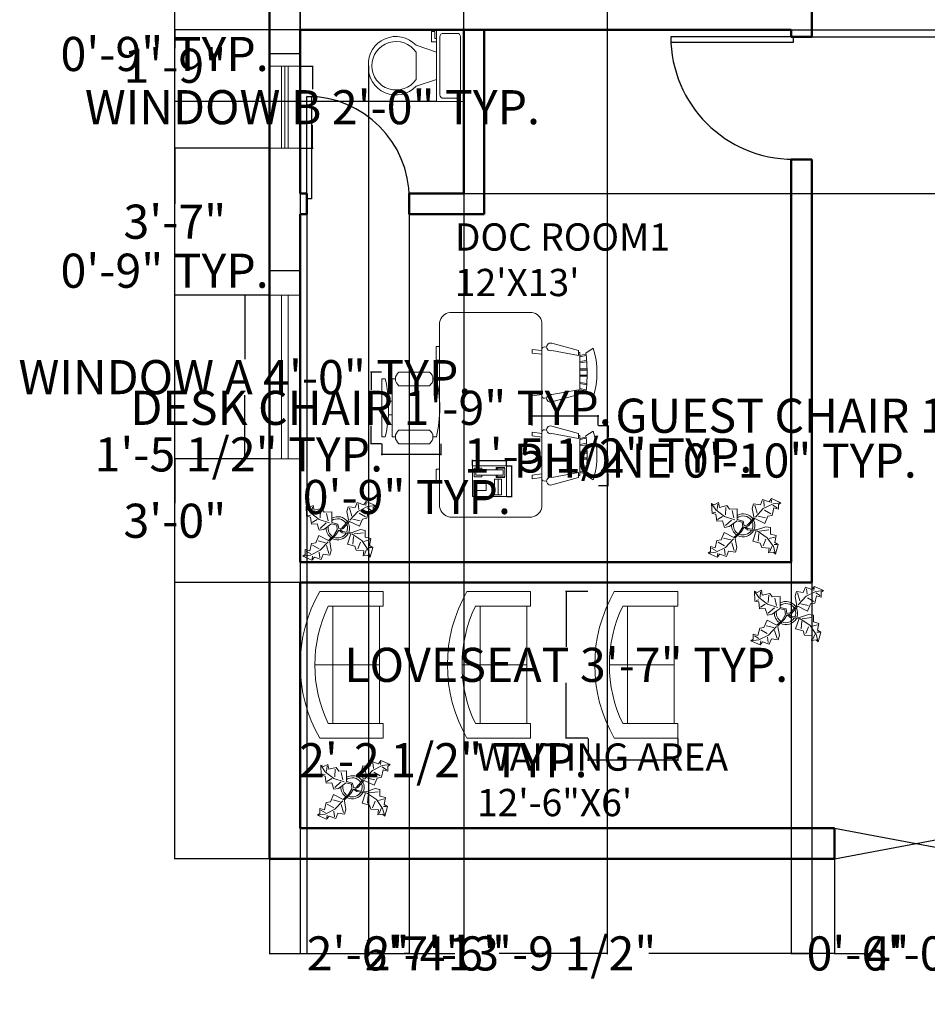
# Model space of a CAD drawing. Units: inches. Extents: x 69 to 644, y 258 to 887.
# Tile 1 of 3: x 69 to 335, y 258 to 546. Entities that reach past the tile are written whole.
import ezdxf

# ---------------------------------------------------------------- set-up
doc = ezdxf.new("R2010")
doc.units = ezdxf.units.IN
doc.header["$MEASUREMENT"] = 0
for name, color, linetype, lineweight in [('A-ANNO-DIMS', 2, 'Continuous', 18), ('A-AREA-IDEN', 7, 'Continuous', 25), ('A-DOOR', 4, 'Continuous', 25), ('A-EQPM', 8, 'Continuous', 13), ('A-FLOR-FIXT', 9, 'Continuous', 18), ('A-FURN', 8, 'Continuous', 18), ('A-GLAZ', 4, 'Continuous', 18), ('A-WALL', 7, 'Continuous', 50), ('PLANT', 3, 'Continuous', 13)]:
    doc.layers.add(name, color=color, linetype=linetype, lineweight=lineweight)
doc.styles.get("Standard").update_dxf_attribs({"font": 'arial.ttf'})
doc.dimstyles.get("Standard").update_dxf_attribs({"dimtxt": 10, "dimasz": 0.18, "dimexe": 0.18, "dimexo": 0.0625, "dimgap": 0.09, "dimtad": 0, "dimtih": 1, "dimtoh": 1, "dimdec": 0, "dimzin": 0, "dimdsep": 46, "dimlunit": 3, "dimtxsty": 'Standard', "dimcen": 0.09, "dimadec": 0, "dimazin": 0, "dimtfac": 1, "dimtdec": 0, "dimtofl": 0, "dimtmove": 0, "dimatfit": 3, "dimfxl": 1, "dimtolj": 1, "dimtzin": 0, "dimarcsym": 0})

# ---------------------------------------------------------------- blocks, each defined once
blk = doc.blocks.new('Phone - Desk')
for p, q in [((-4.5, -5), (-4.5, 5)), ((-4.5, 5), (4.5, 5)), ((-4, 4.5), (-4, 2)), ((-3.75, 4.5), (-3.75, 2.25)), ((-1.25, 4.5), (-3.75, 4.5)), ((-3.25, 4), (-3.25, -4)), ((-3.25, 4), (-1.75, 4)), ((-1.75, -4), (-1.75, 4)), ((-1.25, 2.25), (-1.25, 4.5)), ((-1, 2), (-1, 4.5)), ((4, 3.5), (-0.5, 3.5)), ((-0.5, 3.5), (-0.5, 1.5)), ((4, 1.5), (4, 3.5)), ((4.5, 5), (4.5, -5)), ((-4, 2), (-3.25, 2)), ((-3.75, 2.25), (-3.25, 2.25)), ((-1.75, 2.25), (-1.25, 2.25)), ((-1.75, 2), (-1, 2)), ((-0.5, 2.5), (4, 2.5)), ((-0.5, 1.5), (4, 1.5)), ((-3.75, -2.25), (-3.25, -2.25)), ((-3.75, -4.5), (-3.75, -2.25)), ((-1.75, -2.25), (-1.25, -2.25)), ((-1.25, -2.25), (-1.25, -4.5)), ((2.75, -1), (0.75, -1)), ((0.75, -1), (0.75, -4)), ((2.75, -4), (2.75, -1)), ((4.5, -5), (-4.5, -5)), ((-1.25, -4.5), (-3.75, -4.5)), ((-3.25, -4), (-1.75, -4)), ((0.75, -4), (2.75, -4))]:
    blk.add_line(p, q)
blk = doc.blocks.new('Sofa - Roundback Loveseat 5 ft.')
for p, q in [((0, -32.44198), (0, -5.99998)), ((-24, -33.99998), (-24, -11.46958)), ((24.00004, -33.99998), (24.00004, -11.46958)), ((-23.9998, -13.38178), (23.99986, -13.38178)), ((-24, -32.44198), (24.00004, -32.44198))]:
    blk.add_line(p, q)
for points in [[(-24, -33.99998), (-30, -33.99998), (-30, -7.99998)], [(30.00004, -7.99998), (30.00004, -33.99998), (24.00004, -33.99998)]]:
    blk.add_lwpolyline(points)
for centre, radius, start, end in [((0, -60.24998), 60.24998, 60.13715, 119.8628), ((0, -61.38438), 55.38444, 64.32083, 115.6792)]:
    blk.add_arc(centre, radius, start, end)
blk = doc.blocks.new('Desk - 30 x 60 in.')
for p, q in [((-26.999995, 0), (26.999995, 0)), ((-29.999995, -27), (-29.999995, -3)), ((29.999995, -3), (29.999995, -27)), ((26.999995, -30), (-26.999995, -30)), ((-20.000005, -30), (-20.000005, -31)), ((-20.000005, -31), (-16.000005, -31)), ((-16.000005, -31), (-16.000005, -30)), ((15.999995, -31), (15.999995, -30)), ((19.999995, -31), (15.999995, -31)), ((19.999995, -30), (19.999995, -31))]:
    blk.add_line(p, q)
for centre, start, end in [((-26.499995, -3.5), 98.1301, 171.8699), ((26.499995, -3.5), 8.130102, 81.8699), ((-26.499995, -26.5), 188.1301, 261.8699), ((26.499995, -26.5), 278.1301, 351.8699)]:
    blk.add_arc(centre, 3.535534, start, end)
blk = doc.blocks.new('Chair - Desk')
for p, q in [((-8.5, 0), (-8.5, -1)), ((-8.5, 0), (8.5, 0)), ((8.5, 0), (8.5, -1)), ((-2, -3), (-2, -1.9355)), ((2, -1.9576), (2, -3)), ((-10.5, -5), (-10.5, -14)), ((-8.5, -3), (-8.5, -4)), ((-8.5, -3), (8.5, -3)), ((-6.5, -14), (-6.5, -5)), ((6.5, -5), (6.5, -14)), ((8.5, -3), (8.5, -4)), ((10.5, -14), (10.5, -5)), ((-8.5, -15), (-8.5, -16)), ((8.5, -15), (8.5, -16))]:
    blk.add_line(p, q)
for centre, radius, start, end in [((0, 34.625), 36.625, 256.5803, 283.4197), ((-8.5, -6.5), 2.5, 36.8699, 143.1301), ((8.5, -6.5), 2.5, 36.8699, 143.1301), ((-8.5, -12.5), 2.5, 216.8699, 323.1301), ((8.5, -12.5), 2.5, 216.8699, 323.1301), ((0, 19.625), 36.625, 256.5803, 283.4197)]:
    blk.add_arc(centre, radius, start, end)
blk = doc.blocks.new('Chair - Rocking')
for p, q in [((-8, -4.5), (-10, -1.5)), ((8, -4.5), (10, -1.5)), ((-9, -7.5), (-12, -18.49999)), ((-7, -7.5), (-9, -7.5)), ((-9, -18.49999), (-7, -7.5)), ((-8.23428, -6.99939), (-8.3093, -7.47958)), ((-8.23041, -7), (8.23915, -7)), ((-7.5, -4.5), (-7, -7)), ((-6.5, -7), (-7.02225, -4.43)), ((-4.5, -7), (-4.96674, -4.19951)), ((-4, -7), (-4.40532, -4.16272)), ((-1.5, -4.05012), (-1.5, -7)), ((-1, -7), (-1, -4.05012)), ((1, -7), (1, -4.04655)), ((1.5, -4.05012), (1.5, -7)), ((4, -7), (4.40187, -4.18694)), ((4.5, -7), (4.96761, -4.19437)), ((6.5, -7), (7, -4.4057)), ((7.5, -4.5), (7, -7)), ((7, -7.5), (9, -7.5)), ((9, -18.49999), (7, -7.5)), ((8.31071, -7.48854), (8.23449, -7.00073)), ((9, -7.5), (12, -18.49999)), ((-10.36644, -20.64523), (-10.5, -21.49999)), ((-9, -22.49999), (-9.5, -26.49999)), ((0, -22.49999), (-9.5, -22.49999)), ((-8, -26.49999), (-7.5, -22.49999)), ((0, -22.49999), (9.5, -22.49999)), ((8, -26.49999), (7.5, -22.49999)), ((9, -22.49999), (9.5, -26.49999)), ((10.5, -21.49999), (10.3575, -20.58798)), ((-9.5, -26.49999), (-8, -26.49999)), ((9.5, -26.49999), (8, -26.49999))]:
    blk.add_line(p, q)
for centre, radius, start, end in [((0, -34.08333), 34.08333, 72.93847, 107.0615), ((0, -68.25004), 64.25, 82.84733, 93.92211), ((0, -68.25004), 64.25, 93.92211, 97.15267), ((-10.5, -18.99999), 1.58114, 161.5651, 18.43495), ((10.5, -18.99999), 1.58114, 161.5651, 18.43495), ((-9.5, -21.49999), 1, 180, 270), ((9.5, -21.49999), 1, 270, 0)]:
    blk.add_arc(centre, radius, start, end)
blk = doc.blocks.new('Plant - Rubber or Philodendron')
for p, q in [((-16.2005, 11.4774), (-13.9899, 8.1064)), ((-16.2005, 11.4774), (-14.8639, 10.7964)), ((-16.0159, 6.3329), (-16.2005, 11.4774)), ((-14.8639, 10.7964), (-12.6195, 11.8975)), ((-13.3174, 8.325), (-13.0735, 11.0065)), ((-12.6195, 11.8975), (-12.1909, 9.4345)), ((-12.1909, 9.4345), (-8.3829, 10.3)), ((-8.3829, 10.3), (-7.0549, 8.501)), ((4.6914, 8.8812), (5.3859, 11.2828)), ((5.3859, 11.2828), (8.8871, 10.7908)), ((5.9878, 10.4842), (7.1971, 6.3869)), ((8.8871, 10.7908), (9.9809, 13.4933)), ((9.9809, 13.4933), (13.3837, 12.301)), ((15.3859, 11.3055), (10.3916, 8.7942)), ((10.5828, 12.6946), (10.8893, 9.7953)), ((13.3837, 12.301), (14.68, 13.9039)), ((14.5816, 13.2037), (14.3848, 11.8033)), ((14.68, 13.9039), (19.3848, 11.8146)), ((15.2875, 10.6053), (17.5907, 9.2105)), ((19.3848, 11.8146), (15.3859, 11.3055)), ((19.3848, 11.8146), (18.1868, 10.9119)), ((18.1868, 10.9119), (18.1925, 8.4119)), ((-14.0069, 5.8704), (-16.0159, 6.3329)), ((-15.3434, 6.5514), (-13.9984, 6.9884)), ((-13.5868, 2.2894), (-14.0069, 5.8704)), ((-13.9899, 8.1064), (-9.5434, 4.7185)), ((-8.8369, 9.409), (-9.0894, 5.6095)), ((-7.0549, 8.501), (-3.0284, 8.6941)), ((-4.8529, 4.012), (-5.7184, 7.82)), ((-3.0284, 8.6941), (-3.0709, 3.1041)), ((4.6914, 8.8812), (5.5014, 4.4831)), ((10.3916, 8.7942), (6.2847, 4.4028)), ((14.2977, 6.1031), (10.9934, 7.9956)), ((14.8995, 5.3044), (12.7005, 4.8994)), ((15.7909, 9.1065), (14.8995, 5.3044)), ((18.1925, 8.4119), (15.7909, 9.1065)), ((-10.6784, 2.491), (-13.5868, 2.2894)), ((-13.1329, 3.1804), (-10.6614, 4.727)), ((-9.5858, -0.8715), (-10.6784, 2.491)), ((-9.5434, 4.7185), (-4.1917, 2.9888)), ((-9.1318, 0.0195), (-5.9793, 2.9025)), ((-7.1228, -0.443), (-3.5248, 2.2131)), ((-3.5248, 2.2131), (-3.3011, 2.4355)), ((-3.3011, 2.4355), (-0.5306, 1.7947)), ((-3.0709, 3.1041), (0.0797, 2.3163)), ((-0.5306, 1.7947), (-0.2255, -0.5527)), ((-0.5306, 1.7947), (-0.5306, 1.7947)), ((0.0797, 2.3163), (0.4866, -0.031)), ((0.4866, -0.031), (2.1141, 0.2298)), ((2.1141, 0.2298), (5.4346, 3.9146)), ((6.1032, 3.6844), (2.8262, -0.031)), ((5.4346, 3.9146), (5.5014, 4.4831)), ((11.1089, 1.1958), (6.1032, 3.6844)), ((7.7005, 4.8881), (11.5025, 3.9967)), ((12.7005, 4.8994), (11.1089, 1.1958)), ((-11.3237, -7.2629), (-9.7321, -3.5593)), ((-9.7321, -3.5593), (-4.7264, -6.0479)), ((-7.1228, -0.443), (-9.5858, -0.8715)), ((-2.019, -3.6148), (-4.7264, -6.0479)), ((-4.0579, -6.2781), (-0.9375, -3.1608)), ((-2.019, -3.6148), (-0.2255, -0.5527)), ((-0.9375, -3.1608), (0.5883, -0.8135)), ((0.5883, -0.8135), (2.2447, -2.0916)), ((2.8262, -0.031), (1.3003, -0.5527)), ((1.3003, -0.5527), (2.4193, -1.4655)), ((2.2447, -2.0916), (6.7108, -2.6626)), ((2.4193, -1.4655), (6.895, -2.1175)), ((4.943, -7.9659), (6.7108, -2.6626)), ((11.6605, -0.5413), (6.895, -2.1175)), ((12.3677, -6.1981), (7.219, -2.6772)), ((8.125, -4.0768), (7.7715, -7.9659)), ((8.3544, -2.7453), (13.1973, -2.1704)), ((11.6605, -0.5413), (14.1354, -0.8948)), ((14.1354, -0.8948), (14.1354, -4.4304)), ((14.1354, -4.4304), (16.9638, -5.1375)), ((-14.4141, -11.4699), (-13.5228, -7.6679)), ((-13.5228, -7.6679), (-11.3237, -7.2629)), ((-12.921, -8.4665), (-9.6166, -10.359)), ((-6.3237, -7.2516), (-10.1257, -6.3602)), ((-9.0148, -11.1577), (-4.9047, -6.8122)), ((-4.611, -12.8477), (-5.8203, -8.7504)), ((-4.1246, -6.8466), (-4.0579, -6.2781)), ((-3.3146, -11.2447), (-4.1246, -6.8466)), ((8.8321, -9.0266), (4.943, -7.9659)), ((9.5392, -11.1479), (8.8321, -9.0266)), ((10.2463, -10.4408), (11.6605, -6.9053)), ((15.5496, -10.7943), (12.3677, -6.1981)), ((16.2567, -5.8446), (13.4283, -6.5517)), ((17.3174, -9.7337), (15.9032, -9.7337)), ((16.9638, -5.1375), (16.2567, -8.673)), ((16.2567, -8.673), (18.0245, -9.7337)), ((18.0245, -9.7337), (16.6103, -14.6834)), ((-18.008, -14.1781), (-16.8101, -13.2754)), ((-18.008, -14.1781), (-14.0091, -13.669)), ((-13.3032, -16.2674), (-18.008, -14.1781)), ((-16.8157, -10.7754), (-14.4141, -11.4699)), ((-16.8101, -13.2754), (-16.8157, -10.7754)), ((-13.9107, -12.9688), (-16.2139, -11.574)), ((-14.0091, -13.669), (-9.0148, -11.1577)), ((-12.0069, -14.6645), (-13.3032, -16.2674)), ((-13.2048, -15.5672), (-13.008, -14.1668)), ((-8.6042, -15.8568), (-12.0069, -14.6645)), ((-9.206, -15.0581), (-9.5126, -12.1588)), ((-7.5103, -13.1543), (-8.6042, -15.8568)), ((-4.0092, -13.6463), (-7.5103, -13.1543)), ((-3.3146, -11.2447), (-4.0092, -13.6463)), ((13.4283, -11.5015), (9.5392, -11.1479)), ((13.0748, -13.9763), (13.4283, -11.5015)), ((15.5496, -13.6228), (13.0748, -13.9763)), ((14.8425, -10.7943), (13.7819, -13.2692)), ((16.6103, -14.6834), (15.5496, -10.7943)), ((16.6103, -14.6834), (15.5496, -13.6228))]:
    blk.add_line(p, q)
for centre, radius, start, end in [((0, 0), 6.1275, 34.37569, 120.1028), ((0.0308, 0.1664), 6, 178.6147, 235.1169), ((0.0308, 0.1664), 5, 168.1647, 238.6725), ((-0.0601, -0.2075), 5.2461, 33.82192, 124.9414), ((-0.2664, 0.1682), 5.2775, 338.4094, 20.03007), ((-0.098, 0.1364), 6.1288, 341.2017, 26.09184), ((-0.0234, 0.3825), 6.1492, 242.5812, 331.2714), ((-0.1102, 0.4886), 5.2883, 247.3711, 327.472)]:
    blk.add_arc(centre, radius, start, end)
blk = doc.blocks.new('*U15')
for p, q in [((0, 0), (0, -6)), ((-40, 0), (-40, -6))]:
    blk.add_line(p, q)
blk.add_lwpolyline([(0, 0), (0, 40), (-1.75, 40), (-1.75, 0)], close=True)
blk.add_arc((0, 0), 40, 90, 180)
blk = doc.blocks.new('*U14')
for p, q in [((0, 0), (0, -6)), ((40, 0), (40, -6))]:
    blk.add_line(p, q)
blk.add_lwpolyline([(0, 0), (0, 40), (1.75, 40), (1.75, 0)], close=True)
blk.add_arc((0, 0), 40, 0, 90)
blk = doc.blocks.new('*U17')
for p, q in [((9.5, -6), (9.5, -2)), ((-10, -8.5), (-8, -8.5)), ((-10, -9.5), (-10, -8.5)), ((-8, -8.5), (-8, -8)), ((-7, -8), (-7, -9.5)), ((-4, -8), (-6, -14)), ((4, -8), (6, -14)), ((-7, -9.5), (-10, -9.5)), ((4, -14), (-4, -14))]:
    blk.add_line(p, q)
blk.add_lwpolyline([(10.5, -8), (10.5, 0), (-10.5, 0), (-10.5, -8)], close=True)
for points in [[(-9.5, -2), (-9.5, -6)], [(8.5, -1), (-8.5, -1)], [(-8.5, -7), (8.5, -7)]]:
    blk.add_lwpolyline(points)
for centre, radius, start, end in [((-8.625, -1.875), 0.8839, 81.8699, 188.1301), ((8.625, -1.875), 0.8839, 351.8699, 98.1301), ((-8.625, -6.125), 0.8839, 171.869898, 278.1301), ((8.625, -6.125), 0.8839, 261.8699, 8.1301), ((-0.4772, -19.9188), 8.0953, 133.01722, 273.38), ((0.0374, -19.8731), 7.127, 124.50543, 269.7), ((-0.0373, -19.8731), 7.127, 270.3, 55.4946), ((0.4773, -19.9188), 8.0953, 266.62, 46.9828)]:
    blk.add_arc(centre, radius, start, end)
blk = doc.blocks.new('WIN-48IN')
for p, q in [((9, 48), (0, 48)), ((3.5, 0), (3.5, 48)), ((5.5, 0), (5.5, 48)), ((9, 0), (0, 0))]:
    blk.add_line(p, q)
blk = doc.blocks.new('WIN-24IN')
for p, q in [((0, 0), (0, 9)), ((24, 0), (24, 9)), ((0, 5.5), (24, 5.5)), ((0, 4.5), (24, 4.5)), ((0, 3.5), (24, 3.5))]:
    blk.add_line(p, q)
blk = doc.blocks.new('*D31')
at = {"layer": 'A-ANNO-DIMS', "color": 0, "lineweight": -2, "transparency": 16777216}
for p, q in [((142.2, 465.63), (134.89, 465.63)), ((135.07, 465.45), (135.07, 446.89)), ((135.07, 417.81), (135.07, 436.37)), ((142.2, 417.63), (134.89, 417.63))]:
    blk.add_line(p, q, dxfattribs=at)
at = {"layer": 'A-ANNO-DIMS', "color": 0, "transparency": 16777216}
for points in [[(135.04, 465.45), (135.1, 465.45), (135.07, 465.63)], [(135.04, 417.81), (135.1, 417.81), (135.07, 417.63)]]:
    blk.add_solid(points, dxfattribs=at)
at = {"layer": 'Defpoints', "color": 0, "transparency": 16777216}
for p in [(142.27, 465.63), (135.07, 417.63), (142.27, 417.63)]:
    blk.add_point(p, dxfattribs=at)
at = {"layer": 'A-ANNO-DIMS', "color": 0, "transparency": 16777216, "insert": (135.07, 441.63), "char_height": 10, "attachment_point": 5}
blk.add_mtext('\\A1;WINDOW A 4\'-0" TYP.', dxfattribs=at)
blk = doc.blocks.new('*D32')
at = {"layer": 'A-ANNO-DIMS', "color": 0, "lineweight": -2, "transparency": 16777216}
for p, q in [((142.27, 472.83), (142.09, 472.83)), ((142.27, 465.69), (142.27, 473.01)), ((151.09, 472.83), (142.45, 472.83)), ((151.27, 465.69), (151.27, 473.01))]:
    blk.add_line(p, q, dxfattribs=at)
at = {"layer": 'A-ANNO-DIMS', "color": 0, "transparency": 16777216}
for points in [[(142.45, 472.86), (142.45, 472.8), (142.27, 472.83)], [(151.09, 472.86), (151.09, 472.8), (151.27, 472.83)]]:
    blk.add_solid(points, dxfattribs=at)
at = {"layer": 'Defpoints', "color": 0, "transparency": 16777216}
for p in [(142.27, 472.83), (142.27, 465.63), (151.27, 465.63)]:
    blk.add_point(p, dxfattribs=at)
at = {"layer": 'A-ANNO-DIMS', "color": 0, "transparency": 16777216, "insert": (111.52, 472.83), "char_height": 10, "attachment_point": 5}
blk.add_mtext('\\A1;0\'-9" TYP.', dxfattribs=at)
blk = doc.blocks.new('*D33')
at = {"layer": 'A-ANNO-DIMS', "color": 0, "lineweight": -2, "transparency": 16777216}
for p, q in [((151.33, 532.77), (155.05, 532.77)), ((154.87, 532.59), (154.87, 526.03)), ((154.87, 508.95), (154.87, 515.5)), ((151.33, 508.77), (155.05, 508.77))]:
    blk.add_line(p, q, dxfattribs=at)
at = {"layer": 'A-ANNO-DIMS', "color": 0, "transparency": 16777216}
for points in [[(154.84, 532.59), (154.9, 532.59), (154.87, 532.77)], [(154.84, 508.95), (154.9, 508.95), (154.87, 508.77)]]:
    blk.add_solid(points, dxfattribs=at)
at = {"layer": 'Defpoints', "color": 0, "transparency": 16777216}
for p in [(151.27, 532.77), (154.87, 532.77), (151.27, 508.77)]:
    blk.add_point(p, dxfattribs=at)
at = {"layer": 'A-ANNO-DIMS', "color": 0, "transparency": 16777216, "insert": (154.87, 520.77), "char_height": 10, "attachment_point": 5}
blk.add_mtext('\\A1;WINDOW B 2\'-0" TYP.', dxfattribs=at)
blk = doc.blocks.new('*D34')
at = {"layer": 'A-ANNO-DIMS', "color": 0, "lineweight": -2, "transparency": 16777216}
for p, q in [((142.27, 536.37), (142.09, 536.37)), ((142.27, 532.83), (142.27, 536.55)), ((151.09, 536.37), (142.45, 536.37)), ((151.27, 532.83), (151.27, 536.55))]:
    blk.add_line(p, q, dxfattribs=at)
at = {"layer": 'A-ANNO-DIMS', "color": 0, "transparency": 16777216}
for points in [[(142.45, 536.4), (142.45, 536.34), (142.27, 536.37)], [(151.09, 536.4), (151.09, 536.34), (151.27, 536.37)]]:
    blk.add_solid(points, dxfattribs=at)
at = {"layer": 'Defpoints', "color": 0, "transparency": 16777216}
for p in [(142.27, 536.37), (142.27, 532.77), (151.27, 532.77)]:
    blk.add_point(p, dxfattribs=at)
at = {"layer": 'A-ANNO-DIMS', "color": 0, "transparency": 16777216, "insert": (111.52, 536.37), "char_height": 10, "attachment_point": 5}
blk.add_mtext('\\A1;0\'-9" TYP.', dxfattribs=at)
blk = doc.blocks.new('*D35')
at = {"layer": 'A-ANNO-DIMS', "color": 0, "lineweight": -2, "transparency": 16777216}
for p, q in [((219.29, 427.48), (219.29, 430.5)), ((219.47, 430.32), (238.47, 430.32)), ((238.65, 427.48), (238.65, 430.5)), ((238.65, 430.32), (238.83, 430.32))]:
    blk.add_line(p, q, dxfattribs=at)
at = {"layer": 'A-ANNO-DIMS', "color": 0, "transparency": 16777216}
for points in [[(219.47, 430.35), (219.47, 430.29), (219.29, 430.32)], [(238.47, 430.35), (238.47, 430.29), (238.65, 430.32)]]:
    blk.add_solid(points, dxfattribs=at)
at = {"layer": 'Defpoints', "color": 0, "transparency": 16777216}
for p in [(238.65, 430.32), (219.29, 427.41), (238.65, 427.41)]:
    blk.add_point(p, dxfattribs=at)
at = {"layer": 'A-ANNO-DIMS', "color": 0, "transparency": 16777216, "insert": (330.64, 430.32), "char_height": 10, "attachment_point": 5}
blk.add_mtext('\\A1;GUEST CHAIR 1\'-7 1/2" TYP.', dxfattribs=at)
blk = doc.blocks.new('*D36')
at = {"layer": 'A-ANNO-DIMS', "color": 0, "lineweight": -2, "transparency": 16777216}
for p, q in [((238.71, 427.41), (241.73, 427.41)), ((241.55, 427.23), (241.55, 423.92)), ((241.55, 410.08), (241.55, 413.39)), ((238.71, 409.9), (241.73, 409.9))]:
    blk.add_line(p, q, dxfattribs=at)
at = {"layer": 'A-ANNO-DIMS', "color": 0, "transparency": 16777216}
for points in [[(241.52, 427.23), (241.58, 427.23), (241.55, 427.41)], [(241.52, 410.08), (241.58, 410.08), (241.55, 409.9)]]:
    blk.add_solid(points, dxfattribs=at)
at = {"layer": 'Defpoints', "color": 0, "transparency": 16777216}
for p in [(238.65, 427.41), (238.65, 409.9), (241.55, 409.9)]:
    blk.add_point(p, dxfattribs=at)
at = {"layer": 'A-ANNO-DIMS', "color": 0, "transparency": 16777216, "insert": (241.55, 418.66), "char_height": 10, "attachment_point": 5}
blk.add_mtext('\\A1;1\'-5 1/2" TYP.', dxfattribs=at)
blk = doc.blocks.new('*D39')
at = {"layer": 'A-ANNO-DIMS', "color": 0, "lineweight": -2, "transparency": 16777216}
for p, q in [((201.79, 415.74), (201.79, 417.35)), ((201.97, 417.17), (211.61, 417.17)), ((211.79, 415.74), (211.79, 417.35)), ((211.79, 417.17), (211.97, 417.17))]:
    blk.add_line(p, q, dxfattribs=at)
at = {"layer": 'A-ANNO-DIMS', "color": 0, "transparency": 16777216}
for points in [[(201.97, 417.2), (201.97, 417.14), (201.79, 417.17)], [(211.61, 417.2), (211.61, 417.14), (211.79, 417.17)]]:
    blk.add_solid(points, dxfattribs=at)
at = {"layer": 'Defpoints', "color": 0, "transparency": 16777216}
for p in [(211.79, 417.17), (201.79, 415.67), (211.79, 415.67)]:
    blk.add_point(p, dxfattribs=at)
at = {"layer": 'A-ANNO-DIMS', "color": 0, "transparency": 16777216, "insert": (272.95, 417.17), "char_height": 10, "attachment_point": 5}
blk.add_mtext('\\A1;PHONE 0\'-10" TYP.', dxfattribs=at)
blk = doc.blocks.new('*D40')
at = {"layer": 'A-ANNO-DIMS', "color": 0, "lineweight": -2, "transparency": 16777216}
for p, q in [((211.85, 415.67), (213.47, 415.67)), ((213.29, 415.49), (213.29, 406.85)), ((211.85, 406.67), (213.47, 406.67)), ((213.29, 406.49), (213.11, 406.49)), ((213.29, 406.67), (213.29, 406.49))]:
    blk.add_line(p, q, dxfattribs=at)
at = {"layer": 'A-ANNO-DIMS', "color": 0, "transparency": 16777216}
for points in [[(213.26, 415.49), (213.32, 415.49), (213.29, 415.67)], [(213.26, 406.85), (213.32, 406.85), (213.29, 406.67)]]:
    blk.add_solid(points, dxfattribs=at)
at = {"layer": 'Defpoints', "color": 0, "transparency": 16777216}
for p in [(211.79, 415.67), (211.79, 406.67), (213.29, 406.67)]:
    blk.add_point(p, dxfattribs=at)
at = {"layer": 'A-ANNO-DIMS', "color": 0, "transparency": 16777216, "insert": (182.54, 406.49), "char_height": 10, "attachment_point": 5}
blk.add_mtext('\\A1;0\'-9" TYP.', dxfattribs=at)
blk = doc.blocks.new('*D45')
at = {"layer": 'A-ANNO-DIMS', "color": 0, "lineweight": -2, "transparency": 16777216}
for p, q in [((175.15, 443.12), (171.88, 443.12)), ((172.06, 442.94), (172.06, 437.89)), ((172.06, 422.3), (172.06, 427.36)), ((175.15, 422.12), (171.88, 422.12))]:
    blk.add_line(p, q, dxfattribs=at)
at = {"layer": 'A-ANNO-DIMS', "color": 0, "transparency": 16777216}
for points in [[(172.03, 442.94), (172.09, 442.94), (172.06, 443.12)], [(172.03, 422.3), (172.09, 422.3), (172.06, 422.12)]]:
    blk.add_solid(points, dxfattribs=at)
at = {"layer": 'Defpoints', "color": 0, "transparency": 16777216}
for p in [(172.06, 443.12), (175.21, 443.12), (175.21, 422.12)]:
    blk.add_point(p, dxfattribs=at)
at = {"layer": 'A-ANNO-DIMS', "color": 0, "transparency": 16777216, "insert": (172.06, 432.62), "char_height": 10, "attachment_point": 5}
blk.add_mtext('\\A1;DESK CHAIR 1\'-9" TYP.', dxfattribs=at)
blk = doc.blocks.new('*D46')
at = {"layer": 'A-ANNO-DIMS', "color": 0, "lineweight": -2, "transparency": 16777216}
for p, q in [((175.21, 422.06), (175.21, 418.79)), ((192.55, 422.06), (192.55, 418.79)), ((175.21, 418.97), (175.03, 418.97)), ((192.37, 418.97), (175.39, 418.97))]:
    blk.add_line(p, q, dxfattribs=at)
at = {"layer": 'A-ANNO-DIMS', "color": 0, "transparency": 16777216}
for points in [[(175.39, 419), (175.39, 418.94), (175.21, 418.97)], [(192.37, 419), (192.37, 418.94), (192.55, 418.97)]]:
    blk.add_solid(points, dxfattribs=at)
at = {"layer": 'Defpoints', "color": 0, "transparency": 16777216}
for p in [(175.21, 422.12), (192.55, 422.12), (175.21, 418.97)]:
    blk.add_point(p, dxfattribs=at)
at = {"layer": 'A-ANNO-DIMS', "color": 0, "transparency": 16777216, "insert": (133.29, 418.97), "char_height": 10, "attachment_point": 5}
blk.add_mtext('\\A1;1\'-5 1/2" TYP.', dxfattribs=at)
blk = doc.blocks.new('*D47')
at = {"layer": 'A-ANNO-DIMS', "color": 0, "lineweight": -2, "transparency": 16777216}
for p, q in [((235.67, 378.78), (229.1, 378.78)), ((229.28, 378.6), (229.28, 362.54)), ((229.28, 335.95), (229.28, 352.01)), ((235.67, 335.77), (229.1, 335.77))]:
    blk.add_line(p, q, dxfattribs=at)
at = {"layer": 'A-ANNO-DIMS', "color": 0, "transparency": 16777216}
for points in [[(229.25, 378.6), (229.31, 378.6), (229.28, 378.78)], [(229.25, 335.95), (229.31, 335.95), (229.28, 335.77)]]:
    blk.add_solid(points, dxfattribs=at)
at = {"layer": 'Defpoints', "color": 0, "transparency": 16777216}
for p in [(229.28, 378.78), (235.73, 378.78), (235.73, 335.77)]:
    blk.add_point(p, dxfattribs=at)
at = {"layer": 'A-ANNO-DIMS', "color": 0, "transparency": 16777216, "insert": (229.28, 357.28), "char_height": 10, "attachment_point": 5}
blk.add_mtext('\\A1;LOVESEAT 3\'-7" TYP.', dxfattribs=at)
blk = doc.blocks.new('*D48')
at = {"layer": 'A-ANNO-DIMS', "color": 0, "lineweight": -2, "transparency": 16777216}
for p, q in [((235.73, 335.71), (235.73, 329.14)), ((262.01, 335.71), (262.01, 329.14)), ((235.73, 329.32), (235.55, 329.32)), ((261.83, 329.32), (235.91, 329.32))]:
    blk.add_line(p, q, dxfattribs=at)
at = {"layer": 'A-ANNO-DIMS', "color": 0, "transparency": 16777216}
for points in [[(235.91, 329.35), (235.91, 329.29), (235.73, 329.32)], [(261.83, 329.35), (261.83, 329.29), (262.01, 329.32)]]:
    blk.add_solid(points, dxfattribs=at)
at = {"layer": 'Defpoints', "color": 0, "transparency": 16777216}
for p in [(235.73, 335.77), (262.01, 335.77), (235.73, 329.32)]:
    blk.add_point(p, dxfattribs=at)
at = {"layer": 'A-ANNO-DIMS', "color": 0, "transparency": 16777216, "insert": (193.25, 329.32), "char_height": 10, "attachment_point": 5}
blk.add_mtext('\\A1;2\'-2 1/2" TYP.', dxfattribs=at)
blk = doc.blocks.new('*D52')
at = {"layer": 'A-ANNO-DIMS', "color": 0, "lineweight": -2, "transparency": 16777216}
for p, q in [((142.2, 852.42), (114.34, 852.42)), ((114.52, 852.24), (114.52, 581.62)), ((114.52, 300.6), (114.52, 571.22)), ((142.2, 300.42), (114.34, 300.42))]:
    blk.add_line(p, q, dxfattribs=at)
at = {"layer": 'A-ANNO-DIMS', "color": 0, "transparency": 16777216}
for points in [[(114.49, 852.24), (114.55, 852.24), (114.52, 852.42)], [(114.49, 300.6), (114.55, 300.6), (114.52, 300.42)]]:
    blk.add_solid(points, dxfattribs=at)
at = {"layer": 'Defpoints', "color": 0, "transparency": 16777216}
for p in [(114.52, 852.42), (142.27, 852.42), (142.27, 300.42)]:
    blk.add_point(p, dxfattribs=at)
at = {"layer": 'A-ANNO-DIMS', "color": 0, "transparency": 16777216, "insert": (114.52, 576.42), "char_height": 10, "attachment_point": 5}
blk.add_mtext('\\A1;46\'-0"', dxfattribs=at)
blk = doc.blocks.new('*D53')
at = {"layer": 'A-ANNO-DIMS', "color": 0, "lineweight": -2, "transparency": 16777216}
for p, q in [((142.27, 300.36), (142.27, 272.49)), ((307.91, 300.36), (307.91, 272.49)), ((142.45, 272.67), (196.64, 272.67)), ((307.73, 272.67), (253.53, 272.67))]:
    blk.add_line(p, q, dxfattribs=at)
at = {"layer": 'A-ANNO-DIMS', "color": 0, "transparency": 16777216}
for points in [[(142.45, 272.7), (142.45, 272.64), (142.27, 272.67)], [(307.73, 272.7), (307.73, 272.64), (307.91, 272.67)]]:
    blk.add_solid(points, dxfattribs=at)
at = {"layer": 'Defpoints', "color": 0, "transparency": 16777216}
for p in [(142.27, 300.42), (307.91, 300.42), (307.91, 272.67)]:
    blk.add_point(p, dxfattribs=at)
at = {"layer": 'A-ANNO-DIMS', "color": 0, "transparency": 16777216, "insert": (225.09, 272.67), "char_height": 10, "attachment_point": 5}
blk.add_mtext('\\A1;13\'-9 1/2"', dxfattribs=at)
blk = doc.blocks.new('*D54')
at = {"layer": 'A-ANNO-DIMS', "color": 0, "lineweight": -2, "transparency": 16777216}
for p, q in [((307.91, 300.36), (307.91, 272.49)), ((355.91, 300.36), (355.91, 272.49)), ((308.09, 272.67), (318.33, 272.67)), ((355.73, 272.67), (345.49, 272.67))]:
    blk.add_line(p, q, dxfattribs=at)
at = {"layer": 'A-ANNO-DIMS', "color": 0, "transparency": 16777216}
for points in [[(308.09, 272.7), (308.09, 272.64), (307.91, 272.67)], [(355.73, 272.7), (355.73, 272.64), (355.91, 272.67)]]:
    blk.add_solid(points, dxfattribs=at)
at = {"layer": 'Defpoints', "color": 0, "transparency": 16777216}
for p in [(307.91, 300.42), (355.91, 300.42), (355.91, 272.67)]:
    blk.add_point(p, dxfattribs=at)
at = {"layer": 'A-ANNO-DIMS', "color": 0, "transparency": 16777216, "insert": (331.91, 272.67), "char_height": 10, "attachment_point": 5}
blk.add_mtext('\\A1;4\'-0"', dxfattribs=at)
blk = doc.blocks.new('*D58')
at = {"layer": 'A-ANNO-DIMS', "color": 0, "lineweight": -2, "transparency": 16777216}
for p, q in [((295.27, 387.36), (295.27, 272.49)), ((301.27, 381.36), (301.27, 272.49)), ((295.45, 272.67), (301.09, 272.67)), ((301.27, 272.67), (301.45, 272.67))]:
    blk.add_line(p, q, dxfattribs=at)
at = {"layer": 'A-ANNO-DIMS', "color": 0, "transparency": 16777216}
for points in [[(295.45, 272.7), (295.45, 272.64), (295.27, 272.67)], [(301.09, 272.7), (301.09, 272.64), (301.27, 272.67)]]:
    blk.add_solid(points, dxfattribs=at)
at = {"layer": 'Defpoints', "color": 0, "transparency": 16777216}
for p in [(295.27, 387.42), (301.27, 381.42), (301.27, 272.67)]:
    blk.add_point(p, dxfattribs=at)
at = {"layer": 'A-ANNO-DIMS', "color": 0, "transparency": 16777216, "insert": (314.83, 272.67), "char_height": 10, "attachment_point": 5}
blk.add_mtext('\\A1;0\'-6"', dxfattribs=at)
blk = doc.blocks.new('*D59')
at = {"layer": 'A-ANNO-DIMS', "color": 0, "lineweight": -2, "transparency": 16777216}
for p, q in [((151.27, 543.48), (151.27, 880.35)), ((151.45, 880.17), (161.68, 880.17)), ((199.09, 880.17), (188.85, 880.17)), ((199.27, 543.48), (199.27, 880.35))]:
    blk.add_line(p, q, dxfattribs=at)
at = {"layer": 'A-ANNO-DIMS', "color": 0, "transparency": 16777216}
for points in [[(151.45, 880.2), (151.45, 880.14), (151.27, 880.17)], [(199.09, 880.2), (199.09, 880.14), (199.27, 880.17)]]:
    blk.add_solid(points, dxfattribs=at)
at = {"layer": 'Defpoints', "color": 0, "transparency": 16777216}
for p in [(199.27, 880.17), (151.27, 543.42), (199.27, 543.42)]:
    blk.add_point(p, dxfattribs=at)
at = {"layer": 'A-ANNO-DIMS', "color": 0, "transparency": 16777216, "insert": (175.27, 880.17), "char_height": 10, "attachment_point": 5}
blk.add_mtext('\\A1;4\'-0"', dxfattribs=at)
blk = doc.blocks.new('*D60')
at = {"layer": 'A-ANNO-DIMS', "color": 0, "lineweight": -2, "transparency": 16777216}
for p, q in [((199.33, 543.42), (590.2, 543.42)), ((590.02, 543.24), (590.02, 524.62)), ((590.02, 495.6), (590.02, 514.22)), ((199.33, 495.42), (590.2, 495.42))]:
    blk.add_line(p, q, dxfattribs=at)
at = {"layer": 'A-ANNO-DIMS', "color": 0, "transparency": 16777216}
for points in [[(589.99, 543.24), (590.05, 543.24), (590.02, 543.42)], [(589.99, 495.6), (590.05, 495.6), (590.02, 495.42)]]:
    blk.add_solid(points, dxfattribs=at)
at = {"layer": 'Defpoints', "color": 0, "transparency": 16777216}
for p in [(199.27, 543.42), (199.27, 495.42), (590.02, 495.42)]:
    blk.add_point(p, dxfattribs=at)
at = {"layer": 'A-ANNO-DIMS', "color": 0, "transparency": 16777216, "insert": (590.02, 519.42), "char_height": 10, "attachment_point": 5}
blk.add_mtext('\\A1;4\'-0"', dxfattribs=at)
blk = doc.blocks.new('*D61')
at = {"layer": 'A-ANNO-DIMS', "color": 0, "lineweight": -2, "transparency": 16777216}
for p, q in [((153.27, 489.36), (153.27, 272.49)), ((183.27, 489.36), (183.27, 272.49)), ((153.45, 272.67), (154.8, 272.67)), ((183.09, 272.67), (181.73, 272.67))]:
    blk.add_line(p, q, dxfattribs=at)
at = {"layer": 'A-ANNO-DIMS', "color": 0, "transparency": 16777216}
for points in [[(153.45, 272.7), (153.45, 272.64), (153.27, 272.67)], [(183.09, 272.7), (183.09, 272.64), (183.27, 272.67)]]:
    blk.add_solid(points, dxfattribs=at)
at = {"layer": 'Defpoints', "color": 0, "transparency": 16777216}
for p in [(153.27, 489.42), (183.27, 489.42), (183.27, 272.67)]:
    blk.add_point(p, dxfattribs=at)
at = {"layer": 'A-ANNO-DIMS', "color": 0, "transparency": 16777216, "insert": (168.27, 272.67), "char_height": 10, "attachment_point": 5}
blk.add_mtext('\\A1;2\'-6"', dxfattribs=at)
blk = doc.blocks.new('*D62')
at = {"layer": 'A-ANNO-DIMS', "color": 0, "lineweight": -2, "transparency": 16777216}
for p, q in [((142.2, 417.63), (114.34, 417.63)), ((114.52, 417.45), (114.52, 404.72)), ((114.52, 381.6), (114.52, 394.33)), ((151.2, 381.42), (114.34, 381.42))]:
    blk.add_line(p, q, dxfattribs=at)
at = {"layer": 'A-ANNO-DIMS', "color": 0, "transparency": 16777216}
for points in [[(114.49, 417.45), (114.55, 417.45), (114.52, 417.63)], [(114.49, 381.6), (114.55, 381.6), (114.52, 381.42)]]:
    blk.add_solid(points, dxfattribs=at)
at = {"layer": 'Defpoints', "color": 0, "transparency": 16777216}
for p in [(114.52, 417.63), (142.27, 417.63), (151.27, 381.42)]:
    blk.add_point(p, dxfattribs=at)
at = {"layer": 'A-ANNO-DIMS', "color": 0, "transparency": 16777216, "insert": (114.52, 399.52), "char_height": 10, "attachment_point": 5}
blk.add_mtext('\\A1;3\'-0"', dxfattribs=at)
blk = doc.blocks.new('*D63')
at = {"layer": 'A-ANNO-DIMS', "color": 0, "lineweight": -2, "transparency": 16777216}
for p, q in [((142.2, 508.77), (114.34, 508.77)), ((114.52, 508.59), (114.52, 492.4)), ((114.52, 465.81), (114.52, 482)), ((142.2, 465.63), (114.34, 465.63))]:
    blk.add_line(p, q, dxfattribs=at)
at = {"layer": 'A-ANNO-DIMS', "color": 0, "transparency": 16777216}
for points in [[(114.49, 508.59), (114.55, 508.59), (114.52, 508.77)], [(114.49, 465.81), (114.55, 465.81), (114.52, 465.63)]]:
    blk.add_solid(points, dxfattribs=at)
at = {"layer": 'Defpoints', "color": 0, "transparency": 16777216}
for p in [(114.52, 508.77), (142.27, 508.77), (142.27, 465.63)]:
    blk.add_point(p, dxfattribs=at)
at = {"layer": 'A-ANNO-DIMS', "color": 0, "transparency": 16777216, "insert": (114.52, 487.2), "char_height": 10, "attachment_point": 5}
blk.add_mtext('\\A1;3\'-7"', dxfattribs=at)
blk = doc.blocks.new('*D69')
at = {"layer": 'A-ANNO-DIMS', "color": 0, "lineweight": -2, "transparency": 16777216}
for p, q in [((151.27, 693.36), (151.27, 272.49)), ((241.27, 693.36), (241.27, 272.49)), ((151.45, 272.67), (182.93, 272.67)), ((241.09, 272.67), (209.61, 272.67))]:
    blk.add_line(p, q, dxfattribs=at)
at = {"layer": 'A-ANNO-DIMS', "color": 0, "transparency": 16777216}
for points in [[(151.45, 272.7), (151.45, 272.64), (151.27, 272.67)], [(241.09, 272.7), (241.09, 272.64), (241.27, 272.67)]]:
    blk.add_solid(points, dxfattribs=at)
at = {"layer": 'Defpoints', "color": 0, "transparency": 16777216}
for p in [(151.27, 693.42), (241.27, 693.42), (241.27, 272.67)]:
    blk.add_point(p, dxfattribs=at)
at = {"layer": 'A-ANNO-DIMS', "color": 0, "transparency": 16777216, "insert": (196.27, 272.67), "char_height": 10, "attachment_point": 5}
blk.add_mtext('\\A1;7\'-6"', dxfattribs=at)
blk = doc.blocks.new('*D70')
at = {"layer": 'A-ANNO-DIMS', "color": 0, "lineweight": -2, "transparency": 16777216}
for p, q in [((295.33, 543.42), (590.2, 543.42)), ((590.02, 543.42), (590.02, 543.6)), ((590.02, 543.6), (590.2, 543.6)), ((590.02, 541.6), (590.02, 543.24)), ((295.33, 541.42), (590.2, 541.42))]:
    blk.add_line(p, q, dxfattribs=at)
at = {"layer": 'A-ANNO-DIMS', "color": 0, "transparency": 16777216}
for points in [[(589.99, 543.24), (590.05, 543.24), (590.02, 543.42)], [(589.99, 541.6), (590.05, 541.6), (590.02, 541.42)]]:
    blk.add_solid(points, dxfattribs=at)
at = {"layer": 'Defpoints', "color": 0, "transparency": 16777216}
for p in [(295.27, 543.42), (590.02, 543.42), (295.27, 541.42)]:
    blk.add_point(p, dxfattribs=at)
at = {"layer": 'A-ANNO-DIMS', "color": 0, "transparency": 16777216, "insert": (603.58, 543.6), "char_height": 10, "attachment_point": 5}
blk.add_mtext('\\A1;0\'-2"', dxfattribs=at)
blk = doc.blocks.new('*D71')
at = {"layer": 'A-ANNO-DIMS', "color": 0, "lineweight": -2, "transparency": 16777216}
for p, q in [((191.2, 543.41), (114.34, 543.41)), ((114.52, 543.23), (114.52, 538.11)), ((114.52, 522.59), (114.52, 527.72)), ((191.2, 522.41), (114.34, 522.41))]:
    blk.add_line(p, q, dxfattribs=at)
at = {"layer": 'A-ANNO-DIMS', "color": 0, "transparency": 16777216}
for points in [[(114.49, 543.23), (114.55, 543.23), (114.52, 543.41)], [(114.49, 522.59), (114.55, 522.59), (114.52, 522.41)]]:
    blk.add_solid(points, dxfattribs=at)
at = {"layer": 'Defpoints', "color": 0, "transparency": 16777216}
for p in [(114.52, 543.41), (191.27, 543.41), (191.27, 522.41)]:
    blk.add_point(p, dxfattribs=at)
at = {"layer": 'A-ANNO-DIMS', "color": 0, "transparency": 16777216, "insert": (114.52, 532.91), "char_height": 10, "attachment_point": 5}
blk.add_mtext('\\A1;1\'-9"', dxfattribs=at)
blk = doc.blocks.new('*D72')
at = {"layer": 'A-ANNO-DIMS', "color": 0, "lineweight": -2, "transparency": 16777216}
for p, q in [((171.27, 532.85), (171.27, 272.49)), ((199.27, 522.35), (199.27, 272.49)), ((171.45, 272.67), (171.8, 272.67)), ((199.09, 272.67), (198.73, 272.67))]:
    blk.add_line(p, q, dxfattribs=at)
at = {"layer": 'A-ANNO-DIMS', "color": 0, "transparency": 16777216}
for points in [[(171.45, 272.7), (171.45, 272.64), (171.27, 272.67)], [(199.09, 272.7), (199.09, 272.64), (199.27, 272.67)]]:
    blk.add_solid(points, dxfattribs=at)
at = {"layer": 'Defpoints', "color": 0, "transparency": 16777216}
for p in [(171.27, 532.91), (199.27, 522.41), (199.27, 272.67)]:
    blk.add_point(p, dxfattribs=at)
at = {"layer": 'A-ANNO-DIMS', "color": 0, "transparency": 16777216, "insert": (185.27, 272.67), "char_height": 10, "attachment_point": 5}
blk.add_mtext('\\A1;2\'-4"', dxfattribs=at)

msp = doc.modelspace()

# ---------------------------------------------------------------- linework, layer by layer
at = {"layer": 'A-DOOR'}
for p, q in [((307.91, 309.42), (355.91, 300.42)), ((307.91, 300.42), (355.91, 309.42))]:
    msp.add_line(p, q, dxfattribs=at)
at = {"layer": 'A-WALL'}
for p, q in [((142.27, 300.42), (142.27, 852.42)), ((301.27, 543.42), (301.27, 549.42)), ((151.27, 543.42), (295.27, 543.42)), ((151.27, 495.42), (151.27, 543.42)), ((199.27, 495.42), (199.27, 543.42)), ((205.27, 489.42), (205.27, 543.42)), ((295.27, 541.42), (295.27, 543.42)), ((301.27, 543.42), (301.27, 541.42)), ((301.27, 541.42), (295.27, 541.42)), ((295.27, 387.42), (295.27, 505.42)), ((295.27, 505.42), (301.27, 505.42)), ((301.27, 381.42), (301.27, 505.42)), ((151.27, 495.42), (153.27, 495.42)), ((153.27, 495.42), (153.27, 489.42)), ((183.27, 495.42), (199.27, 495.42)), ((183.27, 489.42), (183.27, 495.42)), ((151.27, 387.42), (151.27, 489.42)), ((153.27, 489.42), (151.27, 489.42)), ((183.27, 489.42), (205.27, 489.42)), ((295.27, 387.42), (151.27, 387.42)), ((151.27, 309.42), (151.27, 381.42)), ((301.27, 381.42), (151.27, 381.42)), ((307.91, 309.42), (151.27, 309.42)), ((307.91, 309.42), (307.91, 300.42)), ((307.91, 300.42), (142.27, 300.42))]:
    msp.add_line(p, q, dxfattribs=at)

# ---------------------------------------------------------------- block references
at = {"layer": 'A-DOOR', "xscale": 0.8980321148011755, "yscale": 0.8980321148011755, "zscale": 0.8980321148011755, "rotation": 90}
msp.add_blockref('*U15', (295.88, 541.42), dxfattribs=at)
at = {"layer": 'A-DOOR', "xscale": 0.7506699854318816, "yscale": 0.7506699854318816, "zscale": 0.7506699854318816}
msp.add_blockref('*U14', (153.27, 493.92), dxfattribs=at)
at = {"layer": 'A-EQPM', "rotation": 270}
msp.add_blockref('Phone - Desk', (206.79, 411.17), dxfattribs=at)
at = {"layer": 'A-FLOR-FIXT', "rotation": 270}
msp.add_blockref('*U17', (199.27, 532.91), dxfattribs=at)
at = {"layer": 'A-FURN'}
for name, p, rotation in [('Desk - 30 x 60 in.', (222.16, 430.62), 270), ('Chair - Desk', (175.21, 432.62), 89.99999999999999)]:
    msp.add_blockref(name, p, dxfattribs=dict(at, rotation=rotation))
at = {"layer": 'A-FURN', "xscale": 0.716801753801156, "yscale": 0.716801753801156, "zscale": 0.716801753801156}
for name, p, rotation in [('Chair - Rocking', (238.29, 442.95), 270), ('Chair - Rocking', (238.29, 418.66), 270), ('Sofa - Roundback Loveseat 5 ft.', (151.27, 357.28), 90), ('Sofa - Roundback Loveseat 5 ft.', (194.45, 357.28), 90), ('Sofa - Roundback Loveseat 5 ft.', (237.64, 357.28), 90)]:
    msp.add_blockref(name, p, dxfattribs=dict(at, rotation=rotation))
at = {"layer": 'A-GLAZ'}
for name, p, rotation in [('WIN-24IN', (151.27, 508.77), 89.99999999999994), ('WIN-48IN', (151.27, 465.63), 180)]:
    msp.add_blockref(name, p, dxfattribs=dict(at, rotation=rotation))
at = {"layer": 'PLANT', "xscale": 0.5698547619027642, "yscale": 0.5698547619027642, "zscale": 0.5698547619027642}
for p in [(162.3, 397.22), (281.16, 398.08), (293.72, 372.37), (166.6, 321.29)]:
    msp.add_blockref('Plant - Rubber or Philodendron', p, dxfattribs=at)

# ---------------------------------------------------------------- texts
at = {"layer": 'A-AREA-IDEN', "char_height": 8, "attachment_point": 1}
for s, width, heights, insert in [("DOC ROOM1\\P12'X13'", 77.0373, [44.4], (196.64, 486.71)), ('WAITING AREA\\P12\'-6"X6\'', 89.8139, [27.52], (203.12, 334.24))]:
    msp.add_mtext_dynamic_manual_height_columns(s, width=width, gutter_width=1, heights=heights, dxfattribs=dict(at, insert=insert))

# ---------------------------------------------------------------- dimensions: what is measured, and where the dimension line sits
at = {"layer": 'A-ANNO-DIMS'}
for base, p1, p2, picture, middle in [((199.27, 880.17), (151.27, 543.42), (199.27, 543.42), '*D59', (175.27, 880.17)), ((241.27, 272.67), (151.27, 693.42), (241.27, 693.42), '*D69', (196.27, 272.67)), ((199.27, 272.67), (171.27, 532.91), (199.27, 522.41), '*D72', (185.27, 272.67)), ((183.27, 272.67), (153.27, 489.42), (183.27, 489.42), '*D61', (168.27, 272.67)), ((301.27, 272.67), (295.27, 387.42), (301.27, 381.42), '*D58', (314.83, 272.67)), ((307.91, 272.67), (142.27, 300.42), (307.91, 300.42), '*D53', (225.09, 272.67)), ((355.91, 272.67), (307.91, 300.42), (355.91, 300.42), '*D54', (331.91, 272.67))]:
    dim = msp.add_linear_dim(base=base, p1=p1, p2=p2, dimstyle='Standard', override={"dimdec": 1, "dimlfac": 1, "dimrnd": 0, "dimzin": 1, "dimdsep": 46, "dimlunit": 4, "dimfrac": 2}, dxfattribs=at)
    dim.commit()
    dim.dimension.update_dxf_attribs({"geometry": picture, "text_midpoint": middle})
for base, p1, p2, picture, middle in [((114.52, 852.42), (142.27, 300.42), (142.27, 852.42), '*D52', (114.52, 576.42)), ((590.02, 543.42), (295.27, 541.42), (295.27, 543.42), '*D70', (603.58, 543.6)), ((114.52, 543.41), (191.27, 522.41), (191.27, 543.41), '*D71', (114.52, 532.91)), ((590.02, 495.42), (199.27, 543.42), (199.27, 495.42), '*D60', (590.02, 519.42)), ((114.52, 508.77), (142.27, 465.63), (142.27, 508.77), '*D63', (114.52, 487.2)), ((114.52, 417.63), (151.27, 381.42), (142.27, 417.63), '*D62', (114.52, 399.52))]:
    dim = msp.add_linear_dim(base=base, p1=p1, p2=p2, angle=90, dimstyle='Standard', override={"dimdec": 1, "dimlfac": 1, "dimrnd": 0, "dimzin": 1, "dimdsep": 46, "dimlunit": 4, "dimfrac": 2}, dxfattribs=at)
    dim.commit()
    dim.dimension.update_dxf_attribs({"geometry": picture, "text_midpoint": middle})
for base, p1, p2, angle, text, picture, middle in [((154.87, 532.77), (151.27, 508.77), (151.27, 532.77), 90, 'WINDOW B <> TYP.', '*D33', (154.87, 520.77)), ((142.27, 536.37), (151.27, 532.77), (142.27, 532.77), 180, '<> TYP.', '*D34', (111.52, 536.37)), ((142.27, 472.83), (151.27, 465.63), (142.27, 465.63), 180, '<> TYP.', '*D32', (111.52, 472.83)), ((135.07, 417.63), (142.27, 465.63), (142.27, 417.63), 270, 'WINDOW A <> TYP.', '*D31', (135.07, 441.63)), ((172.06, 443.12), (175.21, 422.12), (175.21, 443.12), 90, 'DESK CHAIR <> TYP.', '*D45', (172.06, 432.62)), ((175.21, 418.97), (192.55, 422.12), (175.21, 422.12), 180, '<> TYP.', '*D46', (133.29, 418.97)), ((241.55, 409.9), (238.65, 427.41), (238.65, 409.9), 270, '<> TYP.', '*D36', (241.55, 418.66)), ((213.29, 406.67), (211.79, 415.67), (211.79, 406.67), 270, '<> TYP.', '*D40', (182.54, 406.49)), ((229.28, 378.78), (235.73, 335.77), (235.73, 378.78), 90, 'LOVESEAT <> TYP.', '*D47', (229.28, 357.28)), ((235.73, 329.32), (262.01, 335.77), (235.73, 335.77), 180, '<> TYP.', '*D48', (193.25, 329.32))]:
    dim = msp.add_linear_dim(base=base, p1=p1, p2=p2, angle=angle, text=text, dimstyle='Standard', override={"dimdec": 1, "dimlfac": 1, "dimrnd": 0, "dimzin": 1, "dimdsep": 46, "dimlunit": 4, "dimfrac": 2}, dxfattribs=at)
    dim.commit()
    dim.dimension.update_dxf_attribs({"geometry": picture, "text_midpoint": middle})
for base, p1, p2, text, picture, middle in [((238.65, 430.32), (219.29, 427.41), (238.65, 427.41), 'GUEST CHAIR <> TYP.', '*D35', (330.64, 430.32)), ((211.79, 417.17), (201.79, 415.67), (211.79, 415.67), 'PHONE <> TYP.', '*D39', (272.95, 417.17))]:
    dim = msp.add_linear_dim(base=base, p1=p1, p2=p2, text=text, dimstyle='Standard', override={"dimdec": 1, "dimlfac": 1, "dimrnd": 0, "dimzin": 1, "dimdsep": 46, "dimlunit": 4, "dimfrac": 2}, dxfattribs=at)
    dim.commit()
    dim.dimension.update_dxf_attribs({"geometry": picture, "text_midpoint": middle})

doc.saveas('drawing.dxf')
